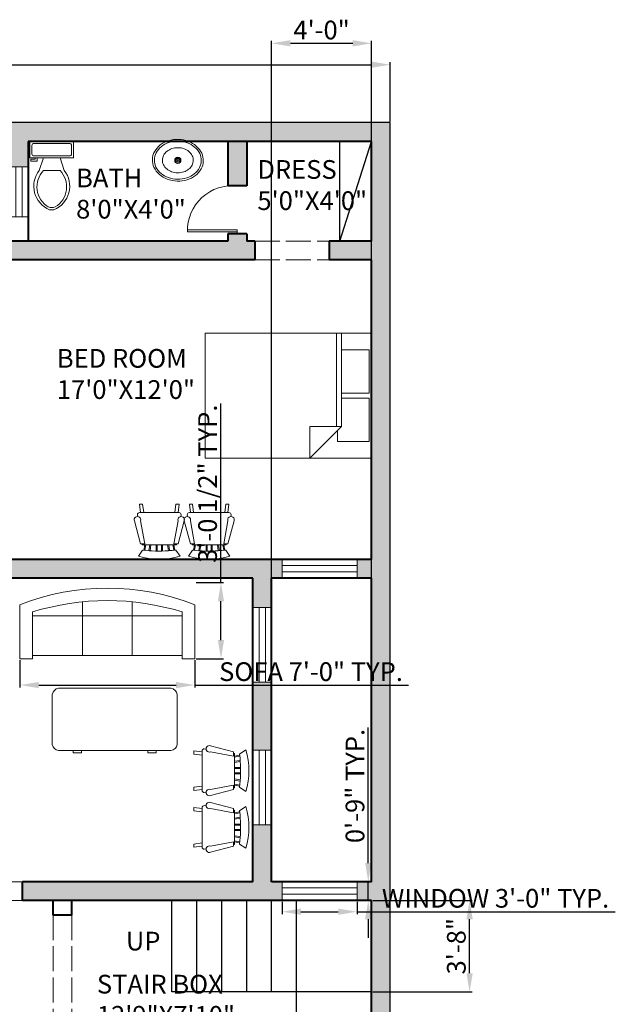
# Model space of a CAD drawing. Units: inches. Extents: x 1967493 to 1968177, y 907234 to 908105.
# Tile 5 of 5: x 1967891 to 1968177, y 907576 to 908050. Entities that reach past the tile are written whole.
import ezdxf

# ---------------------------------------------------------------- set-up
doc = ezdxf.new("R2010")
doc.units = ezdxf.units.IN
doc.linetypes.add('ACAD_ISO02W100', pattern=[15, 12, -3])
for name, color, linetype, lineweight in [('A-ANNO-DIMS', 2, 'Continuous', 18), ('A-ANNO-TEXT', 7, 'Continuous', 18), ('A-AREA-IDEN', 7, 'Continuous', 25), ('A-DOOR', 3, 'Continuous', 20), ('A-FLOR-CASE', 9, 'Continuous', 25), ('A-FLOR-FIXT', 9, 'Continuous', 18), ('A-FLOR-STRS', 7, 'Continuous', 25), ('A-FURN', 8, 'Continuous', 18), ('A-GLAZ', 4, 'Continuous', 18), ('A-WALL', 7, 'Continuous', 40), ('A-WALL-OVHD', 7, 'ACAD_ISO02W100', 18), ('C-PROP', 7, 'Continuous', 25)]:
    doc.layers.add(name, color=color, linetype=linetype, lineweight=lineweight)
doc.layers.add('A-WALL-PATT', color=18, linetype='Continuous', lineweight=13, true_color=0x000000)
doc.styles.get("Standard").update_dxf_attribs({"font": 'arial.ttf'})
doc.dimstyles.new('ISO-25', dxfattribs={"dimtxt": 9, "dimasz": 9, "dimexe": 1.25, "dimexo": 0.625, "dimtad": 1, "dimdec": 1, "dimrnd": 9, "dimlunit": 3, "dimtxsty": 'Standard', "dimcen": 2.5, "dimadec": 0, "dimazin": 0, "dimtfac": 1, "dimtdec": 1, "dimtmove": 0, "dimatfit": 3, "dimfxl": 1, "dimarcsym": 0})

# ---------------------------------------------------------------- blocks, each defined once
blk = doc.blocks.new('Toilet - top')
for p, q in [((9.5, -6), (9.5, -2)), ((-10, -8.5), (-8, -8.5)), ((-10, -9.5), (-10, -8.5)), ((-8, -8.5), (-8, -8)), ((-7, -8), (-7, -9.5)), ((-4, -8), (-6, -14)), ((4, -8), (6, -14)), ((-7, -9.5), (-10, -9.5)), ((4, -14), (-4, -14))]:
    blk.add_line(p, q)
blk.add_lwpolyline([(10.5, -8), (10.5, 0), (-10.5, 0), (-10.5, -8)], close=True)
for points in [[(-9.5, -2), (-9.5, -6)], [(8.5, -1), (-8.5, -1)], [(-8.5, -7), (8.5, -7)]]:
    blk.add_lwpolyline(points)
for centre, radius, start, end in [((-8.62, -1.88), 0.884, 81.8699, 188.1301), ((8.62, -1.88), 0.884, 351.8699, 98.1301), ((-8.62, -6.12), 0.884, 171.8699, 278.1301), ((8.62, -6.12), 0.884, 261.8699, 8.1301), ((3.52, -21.58), 12.17, 141.4691, 247.9714), ((4.2, -21.82), 11.33, 136.3677, 238.9468), ((-3.52, -21.58), 12.17, 292.0284, 38.5307), ((-4.2, -21.82), 11.33, 301.053, 43.6321), ((0, -27.88), 4, 245.7318, 294.2682), ((0, -29), 4, 254.8605, 285.1395)]:
    blk.add_arc(centre, radius, start, end)
blk = doc.blocks.new('Bed - Queen')
for p, q in [((0, -80.00003), (0, 0)), ((0, 0), (59.99999, 0)), ((59.99999, 0), (59.99999, -80.00003)), ((7.99999, -1.2), (28.79998, -1.2)), ((7.99999, -14.4), (7.99999, -1.2)), ((28.79998, -1.2), (28.79998, -14.4)), ((31.19999, -1.2), (51.99999, -1.2)), ((31.19999, -14.4), (31.19999, -1.2)), ((51.99999, -1.2), (51.99999, -16.4)), ((0, -14.4), (44.8, -14.4)), ((44.8, -16.8), (0, -16.8)), ((59.99999, -29.6), (44.8, -14.4)), ((44.8, -14.4), (44.8, -29.6)), ((51.99999, -16.4), (46.79936, -16.4)), ((44.8, -29.6), (59.99999, -29.6)), ((59.99999, -80.00003), (0, -80.00003))]:
    blk.add_line(p, q)
blk = doc.blocks.new('Sink - Oval top')
for p, q in [((-1, 0), (1, 0)), ((0, 1), (0, -1))]:
    blk.add_line(p, q)
for points in [[(-12.23, 0.39, 0.117634), (-11.46, -3.36, 0.104469), (-8.88, -6.8, 0.090016), (-5.08, -9.07, 0.08192), (-0.32, -10.02, 0.08192), (4.49, -9.38, 0.090016), (8.42, -7.36, 0.104469), (11.22, -4.09, 0.117634), (12.23, -0.39, 0.117634), (11.46, 3.36, 0.104469), (8.88, 6.8, 0.090016), (5.08, 9.07, 0.08192), (0.32, 10.02, 0.08192), (-4.49, 9.38, 0.090016), (-8.42, 7.36, 0.104469), (-11.22, 4.09, 0.117634)], [(-11.29, 0.16, 0.118622), (-10.52, -3.25, 0.104678), (-8.07, -6.36, 0.089562), (-4.54, -8.37, 0.081185), (-0.13, -9.15, 0.081185), (4.3, -8.49, 0.089562), (7.89, -6.58, 0.104678), (10.42, -3.55, 0.118622), (11.29, -0.16, 0.118622), (10.52, 3.25, 0.104678), (8.07, 6.36, 0.089562), (4.54, 8.37, 0.081185), (0.13, 9.15, 0.081185), (-4.3, 8.49, 0.089562), (-7.89, 6.58, 0.104678), (-10.42, 3.55, 0.118622)], [(-7.42, 0.08, 0.118283), (-6.91, -2.17, 0.104607), (-5.29, -4.21, 0.089718), (-2.97, -5.53, 0.081436), (-0.07, -6.04, 0.081436), (2.84, -5.59, 0.089718), (5.2, -4.33, 0.104607), (6.86, -2.32, 0.118283), (7.42, -0.08, 0.118283), (6.91, 2.17, 0.104607), (5.29, 4.21, 0.089718), (2.97, 5.53, 0.081436), (0.07, 6.04, 0.081436), (-2.84, 5.59, 0.089718), (-5.2, 4.33, 0.104607), (-6.86, 2.32, 0.118283)]]:
    blk.add_lwpolyline(points, format="xyb", close=True)
for radius in [1.5, 1]:
    blk.add_circle((0, 0), radius)
blk = doc.blocks.new('Sofa - Roundback 7 ft.')
for p, q in [((-12.00002, -32.4421), (-12.00003, -6.5971)), ((11.99997, -32.4421), (11.99998, -6.5971)), ((-36.000027, -34), (-36.000027, -11.4696)), ((-35.999844, -13.3819), (35.9998, -13.3819)), ((35.99998, -34), (35.99998, -11.4696)), ((-36.000027, -32.4421), (35.99998, -32.4421))]:
    blk.add_line(p, q)
for points in [[(-36.000027, -34), (-42.000027, -34), (-42.000027, -8)], [(41.99998, -8), (41.99998, -34), (35.99998, -34)]]:
    blk.add_lwpolyline(points)
for centre, radius, start, end in [((0, -114.25), 114.25, 68.43141, 111.5686), ((-0.00001, -127.1968), 121.1968, 72.72033, 107.2797)]:
    blk.add_arc(centre, radius, start, end)
blk = doc.blocks.new('Desk - 30 x 60 in.')
for p, q in [((-26.999995, 0), (26.999995, 0)), ((-29.999995, -27), (-29.999995, -3)), ((29.999995, -3), (29.999995, -27)), ((26.999995, -30), (-26.999995, -30)), ((-20.000005, -30), (-20.000005, -31)), ((-20.000005, -31), (-16.000005, -31)), ((-16.000005, -31), (-16.000005, -30)), ((15.999995, -31), (15.999995, -30)), ((19.999995, -31), (15.999995, -31)), ((19.999995, -30), (19.999995, -31))]:
    blk.add_line(p, q)
for centre, start, end in [((-26.499995, -3.5), 98.1301, 171.8699), ((26.499995, -3.5), 8.130102, 81.8699), ((-26.499995, -26.5), 188.1301, 261.8699), ((26.499995, -26.5), 278.1301, 351.8699)]:
    blk.add_arc(centre, 3.535534, start, end)
blk = doc.blocks.new('Chair - Rocking')
for p, q in [((-8, -4.5), (-10, -1.5)), ((-7.5, -4.5), (-7, -7)), ((-6.5, -7), (-7.02225, -4.43)), ((-4.5, -7), (-4.96674, -4.19951)), ((-4, -7), (-4.40532, -4.16272)), ((-1.5, -4.05012), (-1.5, -7)), ((-1, -7), (-1, -4.05012)), ((1, -7), (1, -4.04655)), ((1.5, -4.05012), (1.5, -7)), ((4, -7), (4.40187, -4.18694)), ((4.5, -7), (4.96761, -4.19437)), ((6.5, -7), (7, -4.4057)), ((7.5, -4.5), (7, -7)), ((8, -4.5), (10, -1.5)), ((-9, -7.5), (-12, -18.49999)), ((-7, -7.5), (-9, -7.5)), ((-9, -18.49999), (-7, -7.5)), ((-8.23428, -6.99939), (-8.3093, -7.47958)), ((-8.23041, -7), (8.23915, -7)), ((7, -7.5), (9, -7.5)), ((9, -18.49999), (7, -7.5)), ((8.31071, -7.48854), (8.23449, -7.00073)), ((9, -7.5), (12, -18.49999)), ((-10.36644, -20.64523), (-10.5, -21.49999)), ((-9, -22.49999), (-9.5, -26.49999)), ((0, -22.49999), (-9.5, -22.49999)), ((-8, -26.49999), (-7.5, -22.49999)), ((0, -22.49999), (9.5, -22.49999)), ((8, -26.49999), (7.5, -22.49999)), ((9, -22.49999), (9.5, -26.49999)), ((10.5, -21.49999), (10.3575, -20.58798)), ((-9.5, -26.49999), (-8, -26.49999)), ((9.5, -26.49999), (8, -26.49999))]:
    blk.add_line(p, q)
for centre, radius, start, end in [((0, -34.08333), 34.08333, 72.93847, 107.0615), ((0, -68.25004), 64.25, 93.92211, 97.15267), ((0, -68.25004), 64.25, 82.84733, 93.92211), ((-10.5, -18.99999), 1.58114, 161.5651, 18.43495), ((10.5, -18.99999), 1.58114, 161.5651, 18.43495), ((-9.5, -21.49999), 1, 180, 270), ((9.5, -21.49999), 1, 270, 0)]:
    blk.add_arc(centre, radius, start, end)
blk = doc.blocks.new('*D11')
at = {"layer": 'A-ANNO-DIMS', "color": 0, "lineweight": -2, "transparency": 16777216}
for p, q in [((1967588.78, 908000.79), (1967588.78, 908029.28)), ((1967597.78, 908028.03), (1968059.78, 908028.03)), ((1968068.78, 908000.79), (1968068.78, 908029.28))]:
    blk.add_line(p, q, dxfattribs=at)
at = {"layer": 'A-ANNO-DIMS', "color": 0, "transparency": 16777216}
for points in [[(1967597.78, 908029.53), (1967597.78, 908026.53), (1967588.78, 908028.03)], [(1968059.78, 908029.53), (1968059.78, 908026.53), (1968068.78, 908028.03)]]:
    blk.add_solid(points, dxfattribs=at)
at = {"layer": 'Defpoints', "color": 0, "transparency": 16777216}
for p in [(1968068.78, 908028.03), (1967588.78, 908000.17), (1968068.78, 908000.17)]:
    blk.add_point(p, dxfattribs=at)
at = {"layer": 'A-ANNO-DIMS', "color": 0, "transparency": 16777216, "insert": (1967828.78, 908033.25), "char_height": 9, "attachment_point": 5}
blk.add_mtext('39\'-9"', dxfattribs=at)
blk = doc.blocks.new('WIN-36IN')
for p, q in [((0, 9), (0, 0)), ((36, 6), (0, 6)), ((36, 9), (36, 0)), ((36, 3), (0, 3))]:
    blk.add_line(p, q)
blk = doc.blocks.new('WIN-24IN')
for p, q in [((0, 24), (9, 24)), ((3, 24), (3, 0)), ((6, 24), (6, 0)), ((0, 0), (9, 0))]:
    blk.add_line(p, q)
blk = doc.blocks.new('*D22')
at = {"layer": 'A-ANNO-DIMS', "color": 0, "lineweight": -2, "transparency": 16777216}
for p, q in [((1968016.82, 907625.54), (1968016.82, 907619.52)), ((1968052.82, 907625.54), (1968052.82, 907619.52)), ((1968025.82, 907620.77), (1968043.82, 907620.77)), ((1968052.82, 907620.77), (1968176.96, 907620.77))]:
    blk.add_line(p, q, dxfattribs=at)
at = {"layer": 'A-ANNO-DIMS', "color": 0, "transparency": 16777216}
for points in [[(1968025.82, 907622.27), (1968025.82, 907619.27), (1968016.82, 907620.77)], [(1968043.82, 907622.27), (1968043.82, 907619.27), (1968052.82, 907620.77)]]:
    blk.add_solid(points, dxfattribs=at)
at = {"layer": 'Defpoints', "color": 0, "transparency": 16777216}
for p in [(1968016.82, 907626.17), (1968052.82, 907626.17), (1968052.82, 907620.77)]:
    blk.add_point(p, dxfattribs=at)
at = {"layer": 'A-ANNO-DIMS', "color": 0, "transparency": 16777216, "insert": (1968119.39, 907626.05), "char_height": 9, "attachment_point": 5}
blk.add_mtext('WINDOW 3\'-0" TYP.', dxfattribs=at)
blk = doc.blocks.new('*D23')
at = {"layer": 'A-ANNO-DIMS', "color": 0, "lineweight": -2, "transparency": 16777216}
for p, q in [((1968058.22, 907644.17), (1968058.22, 907709.28)), ((1968053.45, 907635.17), (1968059.47, 907635.17)), ((1968058.22, 907626.17), (1968058.22, 907635.17)), ((1968053.45, 907626.17), (1968059.47, 907626.17)), ((1968058.22, 907617.17), (1968058.22, 907608.17))]:
    blk.add_line(p, q, dxfattribs=at)
at = {"layer": 'A-ANNO-DIMS', "color": 0, "transparency": 16777216}
for points in [[(1968056.72, 907644.17), (1968059.72, 907644.17), (1968058.22, 907635.17)], [(1968056.72, 907617.17), (1968059.72, 907617.17), (1968058.22, 907626.17)]]:
    blk.add_solid(points, dxfattribs=at)
at = {"layer": 'Defpoints', "color": 0, "transparency": 16777216}
for p in [(1968052.82, 907635.17), (1968058.22, 907635.17), (1968052.82, 907626.17)]:
    blk.add_point(p, dxfattribs=at)
at = {"layer": 'A-ANNO-DIMS', "color": 0, "transparency": 16777216, "insert": (1968053, 907681.22), "char_height": 9, "attachment_point": 5, "rotation": 90}
blk.add_mtext('0\'-9" TYP.', dxfattribs=at)
blk = doc.blocks.new('*D30')
at = {"layer": 'A-ANNO-DIMS', "color": 0, "lineweight": -2, "transparency": 16777216}
for p, q in [((1967890.81, 907741.72), (1967890.81, 907728.5)), ((1967974.81, 907741.72), (1967974.81, 907728.5)), ((1967899.81, 907729.75), (1967965.81, 907729.75)), ((1967974.81, 907729.75), (1968077.6, 907729.75))]:
    blk.add_line(p, q, dxfattribs=at)
at = {"layer": 'A-ANNO-DIMS', "color": 0, "transparency": 16777216}
for points in [[(1967899.81, 907731.25), (1967899.81, 907728.25), (1967890.81, 907729.75)], [(1967965.81, 907731.25), (1967965.81, 907728.25), (1967974.81, 907729.75)]]:
    blk.add_solid(points, dxfattribs=at)
at = {"layer": 'Defpoints', "color": 0, "transparency": 16777216}
for p in [(1967890.81, 907742.35), (1967974.81, 907742.35), (1967974.81, 907729.75)]:
    blk.add_point(p, dxfattribs=at)
at = {"layer": 'A-ANNO-DIMS', "color": 0, "transparency": 16777216, "insert": (1968030.7, 907735.03), "char_height": 9, "attachment_point": 5}
blk.add_mtext('SOFA 7\'-0" TYP.', dxfattribs=at)
blk = doc.blocks.new('*D31')
at = {"layer": 'A-ANNO-DIMS', "color": 0, "lineweight": -2, "transparency": 16777216}
for p, q in [((1967987.41, 907779.01), (1967987.41, 907865.09)), ((1967975.43, 907779.01), (1967988.66, 907779.01)), ((1967987.41, 907751.35), (1967987.41, 907770.01)), ((1967975.43, 907742.35), (1967988.66, 907742.35))]:
    blk.add_line(p, q, dxfattribs=at)
at = {"layer": 'A-ANNO-DIMS', "color": 0, "transparency": 16777216}
for points in [[(1967985.91, 907770.01), (1967988.91, 907770.01), (1967987.41, 907779.01)], [(1967985.91, 907751.35), (1967988.91, 907751.35), (1967987.41, 907742.35)]]:
    blk.add_solid(points, dxfattribs=at)
at = {"layer": 'Defpoints', "color": 0, "transparency": 16777216}
for p in [(1967974.81, 907779.01), (1967987.41, 907779.01), (1967974.81, 907742.35)]:
    blk.add_point(p, dxfattribs=at)
at = {"layer": 'A-ANNO-DIMS', "color": 0, "transparency": 16777216, "insert": (1967982.13, 907826.55), "char_height": 9, "attachment_point": 5, "rotation": 90}
blk.add_mtext('3\'-0 1/2" TYP.', dxfattribs=at)
blk = doc.blocks.new('*D48')
at = {"layer": 'A-ANNO-DIMS', "color": 0, "lineweight": -2, "transparency": 16777216}
for p, q in [((1968011.78, 907635.79), (1968011.78, 908039.57)), ((1968020.78, 908038.32), (1968050.78, 908038.32)), ((1968059.78, 907635.79), (1968059.78, 908039.57))]:
    blk.add_line(p, q, dxfattribs=at)
at = {"layer": 'A-ANNO-DIMS', "color": 0, "transparency": 16777216}
for points in [[(1968020.78, 908039.82), (1968020.78, 908036.82), (1968011.78, 908038.32)], [(1968050.78, 908039.82), (1968050.78, 908036.82), (1968059.78, 908038.32)]]:
    blk.add_solid(points, dxfattribs=at)
at = {"layer": 'Defpoints', "color": 0, "transparency": 16777216}
for p in [(1968059.78, 908038.32), (1968011.78, 907635.17), (1968059.78, 907635.17)]:
    blk.add_point(p, dxfattribs=at)
at = {"layer": 'A-ANNO-DIMS', "color": 0, "transparency": 16777216, "insert": (1968035.78, 908043.54), "char_height": 9, "attachment_point": 5}
blk.add_mtext('4\'-0"', dxfattribs=at)
blk = doc.blocks.new('*D51')
at = {"layer": 'A-ANNO-DIMS', "color": 0, "lineweight": -2, "transparency": 16777216}
for p, q in [((1968060.4, 907626.17), (1968108.18, 907626.17)), ((1968106.93, 907591.17), (1968106.93, 907617.17)), ((1968060.4, 907582.17), (1968108.18, 907582.17))]:
    blk.add_line(p, q, dxfattribs=at)
at = {"layer": 'A-ANNO-DIMS', "color": 0, "transparency": 16777216}
for points in [[(1968105.43, 907617.17), (1968108.43, 907617.17), (1968106.93, 907626.17)], [(1968105.43, 907591.17), (1968108.43, 907591.17), (1968106.93, 907582.17)]]:
    blk.add_solid(points, dxfattribs=at)
at = {"layer": 'Defpoints', "color": 0, "transparency": 16777216}
for p in [(1968059.78, 907626.17), (1968106.93, 907626.17), (1968059.78, 907582.17)]:
    blk.add_point(p, dxfattribs=at)
at = {"layer": 'A-ANNO-DIMS', "color": 0, "transparency": 16777216, "insert": (1968101.71, 907604.17), "char_height": 9, "attachment_point": 5, "rotation": 90}
blk.add_mtext('3\'-8"', dxfattribs=at)

msp = doc.modelspace()

# ---------------------------------------------------------------- hatches: boundary and pattern name
at = {"layer": 'A-WALL-PATT'}
h = msp.add_hatch(color=256, dxfattribs=at)
h.dxf.hatch_style = 1
h.paths.add_polyline_path([(1967597.78, 907991.17), (1967717.78, 907991.17), (1967717.78, 907980.85), (1967726.78, 907980.85), (1967726.78, 907991.17), (1967885.78, 907991.17), (1967885.78, 907978.94), (1967894.78, 907978.94), (1967894.78, 907991.17), (1968059.78, 907991.17), (1968059.78, 907943.17), (1968039.39, 907943.17), (1968039.39, 907934.17), (1968059.78, 907934.17), (1968059.78, 907790.17), (1968052.82, 907790.17), (1968052.82, 907781.17), (1968059.78, 907781.17), (1968059.78, 907635.17), (1968052.82, 907635.17), (1968052.82, 907626.17), (1968059.78, 907626.17), (1968059.78, 907532.17), (1967892.06, 907532.17), (1967892.06, 907523.17), (1967951.97, 907523.17), (1967951.97, 907525.77), (1968004.23, 907525.77), (1968004.23, 907523.17), (1968059.78, 907523.17), (1968059.78, 907280.17), (1968068.78, 907280.17), (1968068.78, 908000.17), (1967588.78, 908000.17), (1967588.78, 907334.17), (1967828.78, 907334.17), (1967828.78, 907349.71), (1967819.78, 907349.71), (1967819.78, 907343.17), (1967597.78, 907343.17), (1967597.78, 907475.17), (1967774.78, 907475.17), (1967774.78, 907487.51), (1967765.78, 907487.51), (1967765.78, 907479.67), (1967597.78, 907479.67), (1967597.78, 907527.67), (1967604.66, 907527.67), (1967604.66, 907532.17), (1967597.78, 907532.17), (1967597.78, 907790.17), (1967597.78, 907934.17), (1967607.68, 907934.17), (1967607.68, 907943.17), (1967597.78, 907943.17)])
h.paths.add_polyline_path([(1967726.78, 907956.85), (1967717.78, 907956.85), (1967717.78, 907943.17), (1967726.78, 907943.17)], flags=17)
h.paths.add_polyline_path([(1967731.77, 907943.17), (1967651.01, 907943.17), (1967639.17, 907943.17), (1967639.17, 907934.17), (1967651.01, 907934.17), (1967731.77, 907934.17)], flags=17)
h.paths.add_polyline_path([(1967810.78, 907895.17), (1967774.78, 907895.17), (1967774.78, 907903.7), (1967765.78, 907903.7), (1967765.78, 907849.82), (1967765.78, 907834.76), (1967774.78, 907834.76), (1967774.78, 907849.82), (1967774.78, 907886.17), (1967810.78, 907886.17)], flags=17)
h.paths.add_polyline_path([(1967855.78, 907903.7), (1967846.78, 907903.7), (1967846.78, 907895.17), (1967845.59, 907895.17), (1967845.59, 907886.17), (1967846.78, 907886.17), (1967846.78, 907849.82), (1967846.78, 907834.76), (1967855.78, 907834.76), (1967855.78, 907849.82)], flags=17)
h.paths.add_polyline_path([(1968003.67, 907943.17), (1967999.78, 907943.17), (1967999.78, 907946.67), (1967990.78, 907946.67), (1967990.78, 907943.17), (1967881.11, 907943.17), (1967881.11, 907934.17), (1968003.67, 907934.17)], flags=17)
h.paths.add_polyline_path([(1967999.78, 907991.17), (1967990.78, 907991.17), (1967990.78, 907969.75, -0.052013), (1967995.28, 907969.73), (1967999.78, 907969.73)], flags=17)
h.paths.add_polyline_path([(1967777.59, 907790.17), (1967774.78, 907790.17), (1967774.78, 907796.26), (1967765.78, 907796.26), (1967765.78, 907790.17), (1967648.78, 907790.17), (1967648.78, 907769.17), (1967597.78, 907769.17), (1967597.78, 907760.17), (1967648.78, 907760.17), (1967648.78, 907749.33), (1967657.78, 907749.33), (1967657.78, 907781.17), (1967765.78, 907781.17), (1967765.78, 907721), (1967774.78, 907721), (1967774.78, 907781.17), (1967777.59, 907781.17)], flags=17)
h.paths.add_polyline_path([(1968016.82, 907790.17), (1967855.78, 907790.17), (1967855.78, 907796.26), (1967846.78, 907796.26), (1967846.78, 907790.17), (1967843.5, 907790.17), (1967843.5, 907781.17), (1967855.78, 907781.17), (1968002.78, 907781.17), (1968002.78, 907767.09), (1968011.78, 907767.09), (1968011.78, 907781.17), (1968016.82, 907781.17)], flags=17)
h.paths.add_polyline_path([(1968011.78, 907731.09), (1968002.78, 907731.09), (1968002.78, 907698.5), (1968011.78, 907698.5)], flags=17)
h.paths.add_polyline_path([(1968011.78, 907662.5), (1968002.78, 907662.5), (1968002.78, 907635.17), (1967892.06, 907635.17), (1967892.06, 907626.17), (1968016.82, 907626.17), (1968016.82, 907635.17), (1968011.78, 907635.17)], flags=17)
h.paths.add_polyline_path([(1967774.78, 907679.04), (1967765.78, 907679.04), (1967765.78, 907673.17), (1967657.78, 907673.17), (1967657.78, 907679.08), (1967648.78, 907679.08), (1967648.78, 907673.17), (1967639.33, 907673.17), (1967639.33, 907664.17), (1967765.78, 907664.17), (1967765.78, 907577.1), (1967768.96, 907577.1, -0.009361), (1967770.28, 907577.1), (1967774.78, 907577.1), (1967774.78, 907626.17), (1967779.99, 907626.17), (1967779.99, 907635.17), (1967774.78, 907635.17)], flags=17)
h.paths.add_polyline_path([(1967603.33, 907673.17), (1967597.78, 907673.17), (1967597.78, 907664.17), (1967603.33, 907664.17)], flags=17)
h.paths.add_polyline_path([(1967774.78, 907540.27), (1967765.78, 907540.27), (1967765.78, 907532.17), (1967644.82, 907532.17), (1967644.82, 907527.67), (1967765.78, 907527.67), (1967765.78, 907522.83), (1967774.78, 907522.83)], flags=17)
h.paths.add_polyline_path([(1967828.78, 907475.17), (1967828.78, 907479.67), (1967828.78, 907523.17), (1967834.39, 907523.17), (1967834.39, 907532.17), (1967828.78, 907532.17), (1967813.83, 907532.17), (1967813.83, 907527.67), (1967819.78, 907527.67), (1967819.78, 907479.67), (1967819.78, 907475.17), (1967819.78, 907388.61), (1967828.78, 907388.61)], flags=17)

# ---------------------------------------------------------------- linework, layer by layer
at = {"layer": 'A-DOOR'}
for p, q in [((1967971.28, 907947.67), (1967971.28, 907948.67)), ((1967971.28, 907948.67), (1967995.28, 907948.67)), ((1967995.28, 907947.67), (1967971.28, 907947.67)), ((1967995.28, 907948.67), (1967995.28, 907947.67)), ((1967995.28, 907946.67), (1967995.28, 907947.67))]:
    msp.add_line(p, q, dxfattribs=at)
msp.add_arc((1967992.96, 907948.17), 21.69, 83.8652, 181.321, dxfattribs=at)
at = {"layer": 'A-FLOR-CASE'}
for q in [(1968044.62, 907991.17), (1968059.78, 907991.17)]:
    msp.add_line((1968044.62, 907943.17), q, dxfattribs=at)
at = {"layer": 'A-FLOR-STRS'}
for p, q in [((1967963.78, 907582.17), (1967963.78, 907626.17)), ((1967975.78, 907582.17), (1967975.78, 907626.17)), ((1967987.78, 907582.17), (1967987.78, 907626.17)), ((1967999.78, 907582.17), (1967999.78, 907626.17)), ((1968011.78, 907582.17), (1968011.78, 907626.17)), ((1968023.78, 907532.17), (1968023.78, 907626.17)), ((1968059.78, 907582.17), (1967963.78, 907582.17))]:
    msp.add_line(p, q, dxfattribs=at)
at = {"layer": 'A-WALL'}
for p, q in [((1968059.78, 907991.17), (1967894.78, 907991.17)), ((1967894.78, 907991.17), (1967894.78, 907943.17)), ((1967990.78, 907991.17), (1967990.78, 907969.73)), ((1967999.78, 907991.17), (1967999.78, 907969.73)), ((1968059.78, 907943.17), (1968059.78, 907991.17)), ((1967999.78, 907969.73), (1967990.78, 907969.73)), ((1967990.78, 907943.17), (1967846.78, 907943.17)), ((1967999.78, 907946.67), (1967990.78, 907946.67)), ((1967990.78, 907946.67), (1967990.78, 907943.17)), ((1967999.78, 907946.67), (1967999.78, 907943.17)), ((1968003.67, 907943.17), (1967999.78, 907943.17)), ((1968003.67, 907943.17), (1968003.67, 907934.17)), ((1968059.78, 907943.17), (1968039.39, 907943.17)), ((1968039.39, 907943.17), (1968039.39, 907934.17)), ((1968003.67, 907934.17), (1967855.78, 907934.17)), ((1968059.78, 907934.17), (1968039.39, 907934.17)), ((1968059.78, 907790.17), (1968059.78, 907934.17)), ((1968059.78, 907790.17), (1967855.78, 907790.17)), ((1968002.78, 907781.17), (1967846.78, 907781.17)), ((1968002.78, 907635.17), (1968002.78, 907781.17)), ((1968059.78, 907781.17), (1968011.78, 907781.17)), ((1968011.78, 907635.17), (1968011.78, 907781.17)), ((1968059.78, 907635.17), (1968059.78, 907781.17)), ((1968002.78, 907635.17), (1967892.06, 907635.17)), ((1967892.06, 907626.17), (1967892.06, 907635.17)), ((1968059.78, 907635.17), (1968011.78, 907635.17)), ((1968059.78, 907626.17), (1967892.06, 907626.17)), ((1967906.78, 907619.12), (1967906.78, 907626.17)), ((1967915.78, 907619.12), (1967915.78, 907626.17)), ((1968059.78, 907532.17), (1968059.78, 907626.17)), ((1967915.78, 907619.12), (1967906.78, 907619.12))]:
    msp.add_line(p, q, dxfattribs=at)
at = {"layer": 'A-WALL-OVHD'}
for p, q in [((1968003.67, 907943.17), (1968039.39, 907943.17)), ((1968003.67, 907934.17), (1968039.39, 907934.17)), ((1967779.99, 907635.17), (1967892.06, 907635.17)), ((1967779.99, 907626.17), (1967892.06, 907626.17)), ((1967906.78, 907619.12), (1967906.78, 907540.81)), ((1967915.78, 907619.12), (1967915.78, 907540.81))]:
    msp.add_line(p, q, dxfattribs=at)
at = {"layer": 'C-PROP'}
for p, q in [((1968068.78, 908000.17), (1967588.78, 908000.17)), ((1968068.78, 907280.17), (1968068.78, 908000.17))]:
    msp.add_line(p, q, dxfattribs=at)

# ---------------------------------------------------------------- block references
at = {"layer": 'A-FLOR-FIXT'}
for name, p in [('Toilet - top', (1967906.08, 907991.17)), ('Sink - Oval top', (1967966.68, 907982.09))]:
    msp.add_blockref(name, p, dxfattribs=at)
at = {"layer": 'A-FURN'}
for name, p, rotation in [('Bed - Queen', (1968059.78, 907898.92), 270), ('Chair - Rocking', (1967957.78, 907790.17), 180), ('Chair - Rocking', (1967981.74, 907790.17), 180), ('Chair - Rocking', (1968000.87, 907688.58), 270), ('Chair - Rocking', (1968000.87, 907661.32), 270)]:
    msp.add_blockref(name, p, dxfattribs=dict(at, rotation=rotation))
for name, p in [('Sofa - Roundback 7 ft.', (1967932.81, 907776.35)), ('Desk - 30 x 60 in.', (1967936.34, 907728.2))]:
    msp.add_blockref(name, p, dxfattribs=at)
at = {"layer": 'A-GLAZ'}
for name, p in [('WIN-24IN', (1967885.78, 907954.94)), ('WIN-36IN', (1968016.82, 907781.17)), ('WIN-36IN', (1968016.82, 907626.17))]:
    msp.add_blockref(name, p, dxfattribs=at)
for p, rotation in [((1968011.78, 907731.09), 90.00000000008718), ((1968011.78, 907662.5), 90.00000000000003)]:
    msp.add_blockref('WIN-36IN', p, dxfattribs=dict(at, rotation=rotation))

# ---------------------------------------------------------------- texts
at = {"layer": 'A-ANNO-TEXT', "insert": (1967941.71, 907611.13), "char_height": 9, "attachment_point": 1}
msp.add_mtext_dynamic_manual_height_columns('UP', width=25.8504, gutter_width=12.5, heights=[0], dxfattribs=at)
at = {"layer": 'A-AREA-IDEN', "char_height": 9, "attachment_point": 1}
for s, width, insert in [('DRESS \\P5\'0"X4\'0"', 56.0747, (1968004.92, 907982.16)), ('BATH\\P8\'0"X4\'0"', 61.8628, (1967917.78, 907978.05)), ('BED ROOM\\P17\'0"X12\'0"', 91.0854, (1967908.54, 907891.33)), ('STAIR BOX\\P12\'9"X7\'10"', 82.0284, (1967927.78, 907590.43))]:
    msp.add_mtext_dynamic_manual_height_columns(s, width=width, gutter_width=12.5, heights=[0], dxfattribs=dict(at, insert=insert))

# ---------------------------------------------------------------- dimensions: what is measured, and where the dimension line sits
at = {"layer": 'A-ANNO-DIMS'}
for base, p1, p2, override, picture, middle in [((1968059.78, 908038.32), (1968011.78, 907635.17), (1968059.78, 907635.17), {"dimdec": 1, "dimlfac": 1, "dimrnd": 0, "dimzin": 1, "dimdsep": 46, "dimlunit": 4, "dimfrac": 2}, '*D48', (1968035.78, 908043.54)), ((1968068.78, 908028.03), (1967588.78, 908000.17), (1968068.78, 908000.17), {"dimclrd": 0, "dimclre": 0, "dimclrt": 0}, '*D11', (1967828.78, 908033.25))]:
    dim = msp.add_linear_dim(base=base, p1=p1, p2=p2, dimstyle='ISO-25', override=override, dxfattribs=at)
    dim.commit()
    dim.dimension.update_dxf_attribs({"geometry": picture, "text_midpoint": middle})
for base, p1, p2, picture, middle in [((1967987.41, 907779.01), (1967974.81, 907742.35), (1967974.81, 907779.01), '*D31', (1967982.13, 907826.55)), ((1968058.22, 907635.17), (1968052.82, 907626.17), (1968052.82, 907635.17), '*D23', (1968053, 907681.22))]:
    dim = msp.add_linear_dim(base=base, p1=p1, p2=p2, angle=90, text='<> TYP.', dimstyle='ISO-25', override={"dimdec": 1, "dimlfac": 1, "dimrnd": 0, "dimzin": 1, "dimdsep": 46, "dimlunit": 4, "dimfrac": 2}, dxfattribs=at)
    dim.commit()
    dim.dimension.update_dxf_attribs({"geometry": picture, "text_midpoint": middle})
for base, p1, p2, text, picture, middle in [((1967974.81, 907729.75), (1967890.81, 907742.35), (1967974.81, 907742.35), 'SOFA <> TYP.', '*D30', (1968030.7, 907735.03)), ((1968052.82, 907620.77), (1968016.82, 907626.17), (1968052.82, 907626.17), 'WINDOW <> TYP.', '*D22', (1968119.39, 907626.05))]:
    dim = msp.add_linear_dim(base=base, p1=p1, p2=p2, text=text, dimstyle='ISO-25', override={"dimdec": 1, "dimlfac": 1, "dimrnd": 0, "dimzin": 1, "dimdsep": 46, "dimlunit": 4, "dimfrac": 2}, dxfattribs=at)
    dim.commit()
    dim.dimension.update_dxf_attribs({"geometry": picture, "text_midpoint": middle})
dim = msp.add_linear_dim(base=(1968106.93, 907626.17), p1=(1968059.78, 907582.17), p2=(1968059.78, 907626.17), angle=90, dimstyle='ISO-25', override={"dimdec": 1, "dimlfac": 1, "dimrnd": 0, "dimzin": 1, "dimdsep": 46, "dimlunit": 4, "dimfrac": 2}, dxfattribs=at)
dim.commit()
dim.dimension.update_dxf_attribs({"geometry": '*D51', "text_midpoint": (1968101.71, 907604.17)})

doc.saveas('drawing.dxf')
